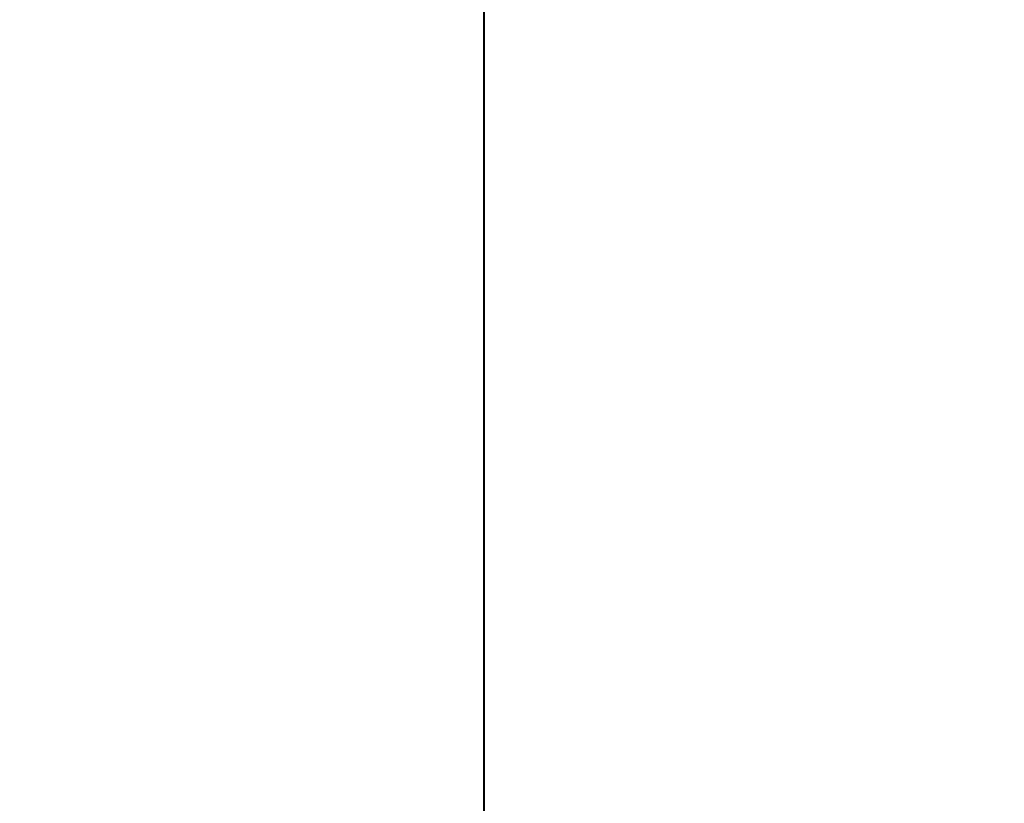
# Model space of a CAD drawing. Units: inches. Extents: x 459864 to 460310, y 324185 to 324787.
# Tile 96 of 112: x 460246.614 to 460247.676, y 324284.275 to 324285.121. Entities that reach past the tile are written whole.
import ezdxf

# ---------------------------------------------------------------- set-up
doc = ezdxf.new("R2010")
doc.units = ezdxf.units.IN
doc.layers.add('A-ANNO-DIMS', color=2, linetype='Continuous', lineweight=18)
doc.layers.add('A-WALL', color=7, linetype='Continuous', lineweight=40)
doc.styles.get("Standard").update_dxf_attribs({"font": 'arial.ttf'})
doc.dimstyles.new('ISO-25', dxfattribs={"dimtxt": 6, "dimasz": 2.5, "dimexe": 1.25, "dimexo": 0.625, "dimtad": 1, "dimdec": 1, "dimlunit": 3, "dimtxsty": 'Standard', "dimcen": 2.5, "dimadec": 0, "dimazin": 0, "dimtfac": 1, "dimtdec": 1, "dimtmove": 0, "dimatfit": 3, "dimfxl": 1, "dimarcsym": 0})

# ---------------------------------------------------------------- blocks, each defined once
blk = doc.blocks.new('*D21')
at = {"layer": 'A-ANNO-DIMS', "color": 0, "lineweight": -2, "transparency": 16777216}
for p, q in [((460247.7399, 324715.4832), (460309.5804, 324715.4832)), ((460308.3304, 324712.9832), (460308.3304, 324285.9832)), ((460247.7399, 324283.4832), (460309.5804, 324283.4832))]:
    blk.add_line(p, q, dxfattribs=at)
at = {"layer": 'A-ANNO-DIMS', "color": 0, "transparency": 16777216}
for points in [[(460307.9137, 324712.9832), (460308.747, 324712.9832), (460308.3304, 324715.4832)], [(460307.9137, 324285.9832), (460308.747, 324285.9832), (460308.3304, 324283.4832)]]:
    blk.add_solid(points, dxfattribs=at)
at = {"layer": 'Defpoints', "color": 0, "transparency": 16777216}
for p in [(460247.1149, 324715.4832), (460247.1149, 324283.4832), (460308.3304, 324283.4832)]:
    blk.add_point(p, dxfattribs=at)
at = {"layer": 'A-ANNO-DIMS', "color": 0, "transparency": 16777216, "insert": (460304.6399, 324499.4832), "char_height": 6, "attachment_point": 5, "rotation": 90}
blk.add_mtext("36'", dxfattribs=at)
blk = doc.blocks.new('*D62')
at = {"layer": 'A-ANNO-DIMS', "color": 0, "lineweight": -2, "transparency": 16777216}
for p, q in [((460247.7399, 324332.7387), (460278.7649, 324332.7387)), ((460277.5149, 324330.2387), (460277.5149, 324285.9832)), ((460247.7399, 324283.4832), (460278.7649, 324283.4832))]:
    blk.add_line(p, q, dxfattribs=at)
at = {"layer": 'A-ANNO-DIMS', "color": 0, "transparency": 16777216}
for points in [[(460277.0983, 324330.2387), (460277.9316, 324330.2387), (460277.5149, 324332.7387)], [(460277.0983, 324285.9832), (460277.9316, 324285.9832), (460277.5149, 324283.4832)]]:
    blk.add_solid(points, dxfattribs=at)
at = {"layer": 'Defpoints', "color": 0, "transparency": 16777216}
for p in [(460247.1149, 324332.7387), (460247.1149, 324283.4832), (460277.5149, 324283.4832)]:
    blk.add_point(p, dxfattribs=at)
at = {"layer": 'A-ANNO-DIMS', "color": 0, "transparency": 16777216, "insert": (460273.7876, 324308.111), "char_height": 6, "attachment_point": 5, "rotation": 90}
blk.add_mtext('4\'-1 1/2"', dxfattribs=at)
blk = doc.blocks.new('*D67')
at = {"layer": 'A-ANNO-DIMS', "color": 0, "lineweight": -2, "transparency": 16777216}
for p, q in [((460208.1149, 324284.1082), (460208.1149, 324315.1332)), ((460247.1149, 324284.1082), (460247.1149, 324315.1332)), ((460210.6149, 324313.8832), (460244.6149, 324313.8832))]:
    blk.add_line(p, q, dxfattribs=at)
at = {"layer": 'A-ANNO-DIMS', "color": 0, "transparency": 16777216}
for points in [[(460210.6149, 324314.2999), (460210.6149, 324313.4666), (460208.1149, 324313.8832)], [(460244.6149, 324314.2999), (460244.6149, 324313.4666), (460247.1149, 324313.8832)]]:
    blk.add_solid(points, dxfattribs=at)
at = {"layer": 'Defpoints', "color": 0, "transparency": 16777216}
for p in [(460247.1149, 324313.8832), (460208.1149, 324283.4832), (460247.1149, 324283.4832)]:
    blk.add_point(p, dxfattribs=at)
at = {"layer": 'A-ANNO-DIMS', "color": 0, "transparency": 16777216, "insert": (460227.6149, 324317.5737), "char_height": 6, "attachment_point": 5}
blk.add_mtext('3\'-3"', dxfattribs=at)

msp = doc.modelspace()

# ---------------------------------------------------------------- linework, layer by layer
at = {"layer": 'A-WALL'}
msp.add_line((460247.1149, 324470.9832), (460247.1149, 324283.4832), dxfattribs=at)

# ---------------------------------------------------------------- dimensions: what is measured, and where the dimension line sits
at = {"layer": 'A-ANNO-DIMS'}
for base, p1, angle, override, picture, middle in [((460308.3304, 324283.4832), (460247.1149, 324715.4832), 90, {"dimclrd": 0, "dimclre": 0, "dimclrt": 0}, '*D21', (460304.6399, 324499.4832)), ((460277.5149, 324283.4832), (460247.1149, 324332.7387), 270, {"dimdec": 1, "dimlfac": 1, "dimrnd": 0, "dimzin": 1, "dimdsep": 46, "dimlunit": 4, "dimfrac": 2}, '*D62', (460273.7876, 324308.111))]:
    dim = msp.add_linear_dim(base=base, p1=p1, p2=(460247.1149, 324283.4832), angle=angle, dimstyle='ISO-25', override=override, dxfattribs=at)
    dim.commit()
    dim.dimension.update_dxf_attribs({"geometry": picture, "text_midpoint": middle})
dim = msp.add_linear_dim(base=(460247.1149, 324313.8832), p1=(460208.1149, 324283.4832), p2=(460247.1149, 324283.4832), dimstyle='ISO-25', override={"dimdec": 1, "dimlfac": 1, "dimrnd": 0, "dimzin": 1, "dimdsep": 46, "dimlunit": 4, "dimfrac": 2}, dxfattribs=at)
dim.commit()
dim.dimension.update_dxf_attribs({"geometry": '*D67', "text_midpoint": (460227.6149, 324317.5737)})

doc.saveas('drawing.dxf')
